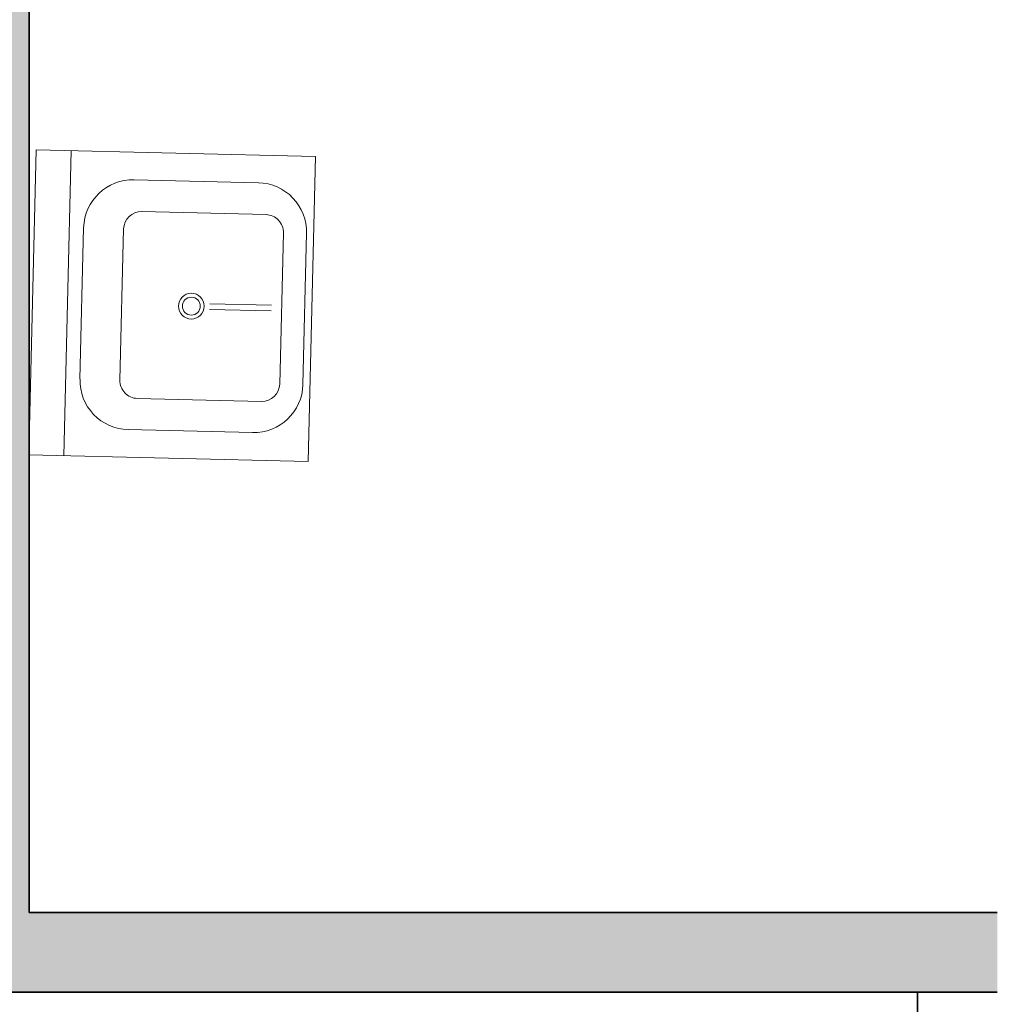
# Model space of a CAD drawing. Units: inches. Extents: x -9 to 505, y -680 to 48.
# Tile 15 of 17: x 124 to 179, y -169 to -114. Entities that reach past the tile are written whole.
import ezdxf

# ---------------------------------------------------------------- set-up
doc = ezdxf.new("R2010")
doc.units = ezdxf.units.IN
doc.header["$MEASUREMENT"] = 0
for name, color, linetype, lineweight in [('A-FLOR-FIXT', 9, 'Continuous', 18), ('A-WALL', 7, 'Continuous', 35), ('A-WALL-PATT', 251, 'Continuous', 13)]:
    doc.layers.add(name, color=color, linetype=linetype, lineweight=lineweight)

# ---------------------------------------------------------------- blocks, each defined once
blk = doc.blocks.new('М14 600х655')
for p, q in [((-655, 600), (-655, 0)), ((-655, 600), (-655, 0)), ((-655, 0), (-655, 600)), ((0, 600), (-655, 600)), ((0, 0), (0, 600)), ((0, 525), (-655, 525)), ((-165.1, 494.1), (-489.9, 494.1)), ((-165.4, 408.4), (-490.2, 408.4)), ((-595.8, 388.1), (-595.8, 121.3)), ((-59.2, 121.3), (-59.2, 388.1)), ((-528.4, 370.1), (-528.4, 103.3)), ((-127.2, 103.3), (-127.2, 370.1)), ((-333.5, 87.1), (-333.5, 219.6)), ((-321.5, 87.1), (-321.5, 219.6)), ((-490.2, 65.1), (-165.4, 65.1)), ((-655, 0), (-655, 0)), ((-655, 0), (-655, 0)), ((-655, 0), (0, 0)), ((-655, 0), (0, 0)), ((-489.9, 15.4), (-165.1, 15.4))]:
    blk.add_line(p, q)
for radius in [27.6, 19.3]:
    blk.add_circle((-327.5, 258.9), radius)
for centre, radius, start, end in [((-489.9, 388.1), 105.9, 90, 180), ((-165.1, 388.1), 105.9, 0, 90), ((-490.2, 370.1), 38.2, 90, 180), ((-165.4, 370.1), 38.2, 0, 90), ((-489.9, 121.3), 105.9, 180, 270), ((-165.1, 121.3), 105.9, 270, 0), ((-490.2, 103.3), 38.2, 180, 270), ((-165.4, 103.3), 38.2, 270, 0)]:
    blk.add_arc(centre, radius, start, end)

msp = doc.modelspace()

# ---------------------------------------------------------------- hatches: boundary and pattern name
at = {"layer": 'A-WALL-PATT'}
h = msp.add_hatch(color=256, dxfattribs=at)
h.dxf.hatch_style = 1
h.paths.add_polyline_path([(101.641, 11.499), (48.264, 11.499), (48.264, 2.499), (72.264, 2.499), (72.264, -21.248), (81.264, -21.248), (81.264, 2.499), (101.641, 2.499)])
h.paths.add_polyline_path([(36.264, 2.499), (27.264, 2.499), (27.264, -6.918), (36.264, -6.918)])
h.paths.add_polyline_path([(81.264, -57.248), (72.264, -57.248), (72.264, -75.501), (81.264, -75.501)])
h.paths.add_polyline_path([(162.764, 11.499), (137.641, 11.499), (137.641, 2.499), (162.764, 2.499)])
h.paths.add_polyline_path([(179.264, 2.499), (174.764, 2.499), (174.764, -75.501), (179.264, -75.501), (179.264, -54.501), (229.514, -54.501), (229.514, -45.501), (179.264, -45.501)])
h.paths.add_polyline_path([(382.256, -45.501), (332.264, -45.501), (332.264, 2.499), (327.764, 2.499), (327.764, -45.501), (277.514, -45.501), (277.514, -54.501), (327.764, -54.501), (327.764, -111.501), (332.264, -111.501), (332.264, -54.501), (382.256, -54.501)])
h.paths.add_polyline_path([(332.264, -128.001), (327.764, -128.001), (327.764, -207.001), (332.264, -207.001)])
h.paths.add_polyline_path([(124.764, -111.501), (36.264, -111.501), (36.264, -116.001), (120.264, -116.001), (120.264, -168.501), (179.264, -168.501), (179.264, -164.001), (124.764, -164.001)])
h.paths.add_polyline_path([(96.264, -164.001), (36.264, -164.001), (36.264, -152.001), (27.264, -152.001), (27.264, -208.879), (36.264, -208.879), (36.264, -168.501), (96.264, -168.501)])
h.paths.add_polyline_path([(36.264, -244.879), (27.264, -244.879), (27.264, -287.001), (36.264, -287.001)])
h.paths.add_polyline_path([(179.264, -204.501), (174.764, -204.501), (174.764, -287.001), (179.264, -287.001)])
h.paths.add_polyline_path([(257.264, -296.001), (248.264, -296.001), (248.264, -446.001), (269.264, -446.001), (269.264, -437.001), (257.264, -437.001)])
h.paths.add_polyline_path([(90.264, -296.001), (81.264, -296.001), (81.264, -348.67), (90.264, -348.67)])
h.paths.add_polyline_path([(90.264, -384.67), (81.264, -384.67), (81.264, -416.001), (90.264, -416.001)])
h.paths.add_polyline_path([(170.264, -452.001), (36.264, -452.001), (36.264, -456.501), (165.764, -456.501), (165.764, -504.501), (165.133, -504.501), (165.133, -509.001), (170.264, -509.001)])
h.paths.add_polyline_path([(141.764, -504.501), (36.264, -504.501), (36.264, -492.501), (27.264, -492.501), (27.264, -565.959), (36.264, -565.959), (36.264, -509.001), (141.764, -509.001)])
h.paths.add_polyline_path([(36.264, -601.959), (27.264, -601.959), (27.264, -658.501), (36.264, -658.501)])
h.paths.add_polyline_path([(170.264, -670.501), (170.264, -634.501), (222.764, -634.501), (222.764, -625.501), (165.764, -625.501), (165.764, -670.501), (36.264, -670.501), (36.264, -679.501), (170.264, -679.501)])
h.paths.add_polyline_path([(332.264, -616.501), (433.894, -616.501), (433.894, -612.001), (332.264, -612.001), (332.264, -610.563), (327.764, -610.563), (327.764, -625.501), (270.764, -625.501), (270.764, -634.501), (327.764, -634.501), (327.764, -658.501), (332.264, -658.501)])
h.paths.add_polyline_path([(459.764, -670.501), (336.764, -670.501), (336.764, -679.501), (459.764, -679.501)])
h.paths.add_polyline_path([(468.764, -545.737), (459.764, -545.737), (459.764, -612.001), (457.894, -612.001), (457.894, -616.501), (459.764, -616.501), (459.764, -658.501), (468.764, -658.501)])
h.paths.add_polyline_path([(332.264, -446.001), (327.764, -446.001), (327.764, -574.563), (332.264, -574.563)])
h.paths.add_polyline_path([(327.764, -437.001), (305.264, -437.001), (305.264, -446.001), (327.764, -446.001)])
h.paths.add_polyline_path([(459.764, -437.001), (348.764, -437.001), (348.764, -446.001), (459.764, -446.001)])
h.paths.add_polyline_path([(468.764, -458.001), (459.764, -458.001), (459.764, -509.737), (468.764, -509.737)])
h.paths.add_polyline_path([(468.764, -365.001), (459.764, -365.001), (459.764, -437.001), (468.764, -437.001)])
h.paths.add_polyline_path([(468.764, -299.601), (459.764, -299.601), (459.764, -344.001), (468.764, -344.001)])
h.paths.add_polyline_path([(468.764, -184.739), (459.764, -184.739), (459.764, -231.001), (401.264, -231.001), (401.264, -235.501), (459.764, -235.501), (459.764, -275.601), (468.764, -275.601)])
h.paths.add_polyline_path([(390.764, -356.001), (342.764, -356.001), (342.764, -365.001), (390.764, -365.001)])
h.paths.add_polyline_path([(459.764, -356.001), (405.764, -356.001), (405.764, -365.001), (459.764, -365.001)])
h.paths.add_polyline_path([(405.764, -296.001), (396.764, -296.001), (396.764, -356.001), (405.764, -356.001)])
h.paths.add_polyline_path([(336.764, -296.001), (327.764, -296.001), (327.764, -356.001), (336.764, -356.001)])
h.paths.add_polyline_path([(468.764, -9.501), (459.764, -9.501), (459.764, -45.501), (418.256, -45.501), (418.256, -54.501), (468.764, -54.501)])
h.paths.add_polyline_path([(468.764, -54.501), (459.764, -54.501), (459.764, -111.501), (468.764, -111.501)])
h.paths.add_polyline_path([(468.764, -128.001), (459.764, -128.001), (459.764, -148.739), (468.764, -148.739)])

# ---------------------------------------------------------------- linework, layer by layer
at = {"layer": 'A-WALL'}
for p, q in [((124.764, -111.501), (124.764, -164.001)), ((124.764, -164.001), (179.264, -164.001)), ((36.264, -168.501), (179.264, -168.501)), ((174.764, -168.501), (174.764, -287.001))]:
    msp.add_line(p, q, dxfattribs=at)

# ---------------------------------------------------------------- block references
at = {"layer": 'A-FLOR-FIXT', "xscale": 0.0262208519320216, "yscale": 0.0262208519320216, "zscale": 0.0262208519320216, "rotation": 88.62400885752176}
msp.add_blockref('М14 600х655', (140.892, -121.454), dxfattribs=at)

doc.saveas('drawing.dxf')
